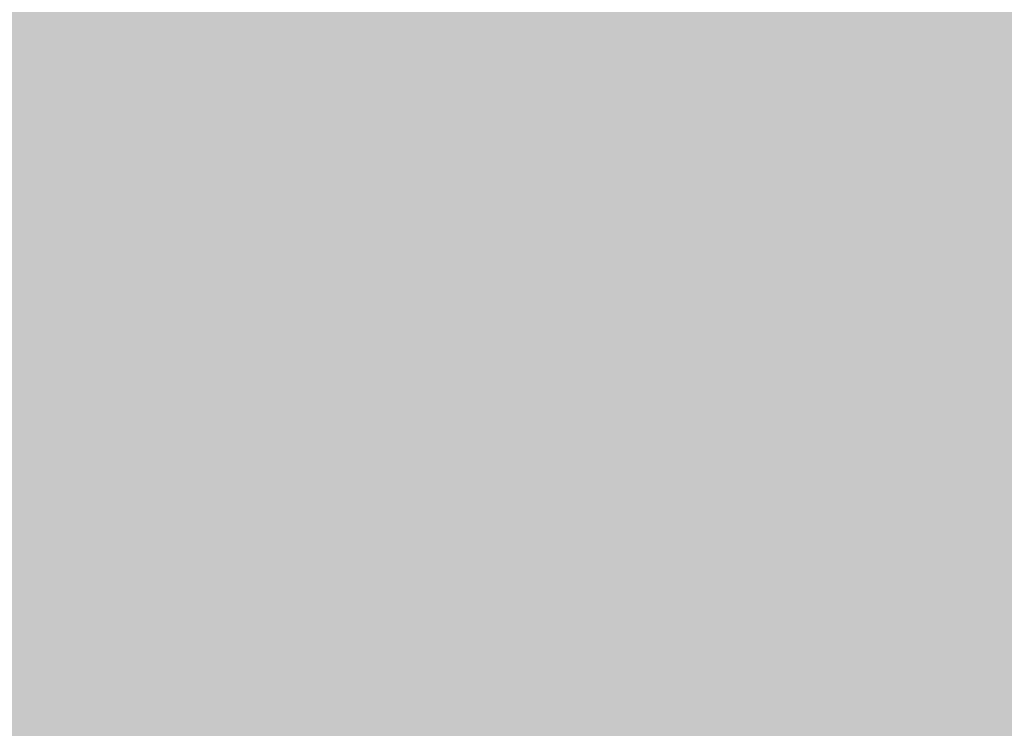
# Model space of a CAD drawing. Units: feet. Extents: x 3168 to 4724, y 827 to 1477.
# Tile 192 of 256: x 3316.07 to 3333.46, y 1074.89 to 1087.4. Entities that reach past the tile are written whole.
import ezdxf

# ---------------------------------------------------------------- set-up
doc = ezdxf.new("R2010")
doc.units = ezdxf.units.FT
doc.layers.add('A-ELEV-PATT', color=8, linetype='Continuous', lineweight=13)

msp = doc.modelspace()

# ---------------------------------------------------------------- hatches: boundary and pattern name
at = {"layer": 'A-ELEV-PATT'}
h = msp.add_hatch(color=256, dxfattribs=at)
h.dxf.hatch_style = 1
edge = h.paths.add_edge_path()
edge.add_ellipse((3552.906, 979.22), major_axis=(36.745, 0), ratio=0.484848, start_angle=0, end_angle=360)
edge = h.paths.add_edge_path()
edge.add_ellipse((3559.892, 929.252), major_axis=(36.745, 0), ratio=0.484848, start_angle=0, end_angle=360)
edge = h.paths.add_edge_path()
edge.add_line((3299.317, 1198.606), (3479.917, 1198.606))
edge.add_line((3479.917, 1198.606), (3479.917, 1209.869))
edge.add_spline(control_points=[(3479.917, 1209.869), (3464.301, 1209.869), (3448.686, 1209.869), (3410.949, 1209.869), (3388.828, 1209.869), (3355.647, 1209.869), (3344.586, 1209.869), (3327.996, 1209.869), (3322.466, 1209.869), (3314.17, 1209.869), (3311.405, 1209.869), (3307.257, 1209.869), (3305.875, 1209.869), (3303.801, 1209.869), (3303.11, 1209.869), (3302.073, 1209.869), (3301.727, 1209.869), (3301.209, 1209.869), (3301.036, 1209.869), (3300.777, 1209.869), (3300.69, 1209.869), (3300.561, 1209.869), (3300.517, 1209.869), (3300.453, 1209.869), (3300.431, 1209.869), (3300.399, 1209.869), (3300.388, 1209.869), (3300.366, 1209.869), (3300.346, 1209.869), (3300.346, 1209.869), (3300.346, 1209.869), (3300.343, 1209.869), (3300.341, 1209.869), (3300.338, 1209.869), (3300.337, 1209.869), (3300.334, 1209.869), (3300.332, 1209.869), (3300.326, 1209.869), (3300.321, 1209.869), (3300.311, 1209.869), (3300.306, 1209.869), (3300.291, 1209.869), (3300.28, 1209.869), (3300.232, 1209.869), (3300.195, 1209.869), (3299.951, 1209.871), (3299.745, 1209.874), (3299.437, 1209.883), (3299.334, 1209.887), (3299.181, 1209.893), (3299.13, 1209.895), (3298.652, 1209.917), (3298.229, 1209.946), (3297.602, 1210.002), (3297.393, 1210.023), (3297.083, 1210.058), (3296.979, 1210.07), (3296.293, 1210.155), (3295.718, 1210.243), (3294.869, 1210.399), (3294.588, 1210.454), (3294.169, 1210.543), (3294.03, 1210.574), (3291.707, 1211.101), (3289.654, 1211.813), (3285.776, 1213.564), (3283.951, 1214.603), (3280.512, 1216.98), (3278.897, 1218.318), (3276.38, 1220.829), (3275.416, 1221.918), (3274.039, 1223.708), (3273.581, 1224.35), (3273.143, 1225.016)], knot_values=[39.119033, 39.119033, 39.119033, 39.119033, 39.286353, 39.286353, 39.523379, 39.523379, 39.641892, 39.641892, 39.701148, 39.701148, 39.730777, 39.730777, 39.745591, 39.745591, 39.752998, 39.752998, 39.756701, 39.756701, 39.758553, 39.758553, 39.759479, 39.759479, 39.759942, 39.759942, 39.760173, 39.760173, 39.760289, 39.760289, 39.760405, 39.760405, 39.760463, 39.760463, 39.763389, 39.763389, 39.764851, 39.764851, 39.767304, 39.767304, 39.773825, 39.773825, 39.78057, 39.78057, 39.79477, 39.79477, 39.845194, 39.845194, 40.126715, 40.126715, 40.267476, 40.267476, 40.337856, 40.337856, 40.927023, 40.927023, 41.221606, 41.221606, 41.368898, 41.368898, 42.202622, 42.202622, 42.619485, 42.619485, 42.827916, 42.827916, 46.118323, 46.118323, 49.408731, 49.408731, 52.699139, 52.699139, 54.927489, 54.927489, 56.104228, 56.104228, 56.104228, 56.104228], weights=[1, 1, 1, 1, 1, 1, 1, 1, 1, 1, 1, 1, 1, 1, 1, 1, 1, 1, 1, 1, 1, 1, 1, 1, 1, 1, 1, 1, 1, 1, 1, 1, 1, 1, 1, 1, 1, 1, 1, 1, 1, 1, 1, 1, 1, 1, 1, 1, 1, 1, 1, 1, 1, 1, 1, 1, 1, 1, 1, 1, 1, 1, 1, 1, 1, 1, 1, 1, 1, 1, 1, 1, 1, 1], degree=3, periodic=0)
edge.add_line((3273.143, 1225.016), (3273.143, 1099.016))
edge.add_line((3273.143, 1099.016), (3299.317, 1099.016))
edge.add_line((3299.317, 1099.016), (3299.317, 1198.606))
edge = h.paths.add_edge_path()
edge.add_line((3304.758, 1324.158), (3479.917, 1324.158))
edge.add_line((3479.917, 1324.158), (3479.917, 1335.715))
edge.add_line((3479.917, 1335.715), (3269.162, 1335.715))
edge.add_spline(control_points=[(3269.162, 1335.715), (3264.024, 1335.715), (3258.364, 1328.958), (3259.264, 1323.9)], knot_values=[0, 0, 0, 0, 15.412191, 15.412191, 15.412191, 15.412191], degree=3, periodic=0)
edge.add_line((3259.264, 1323.9), (3265.517, 1288.769))
edge.add_line((3265.517, 1288.769), (3275.265, 1261.546))
edge.add_line((3275.265, 1261.546), (3304.758, 1261.546))
edge.add_line((3304.758, 1261.546), (3304.758, 1324.158))
h = msp.add_hatch(color=256, dxfattribs=at)
h.dxf.hatch_style = 1
h.paths.add_polyline_path([(3384.525, 1099.016), (3335.029, 1099.016), (3299.317, 1099.016), (3273.143, 1099.016), (3217.565, 1099.016), (3168.069, 827.116), (3335.029, 827.116)])

doc.saveas('drawing.dxf')
